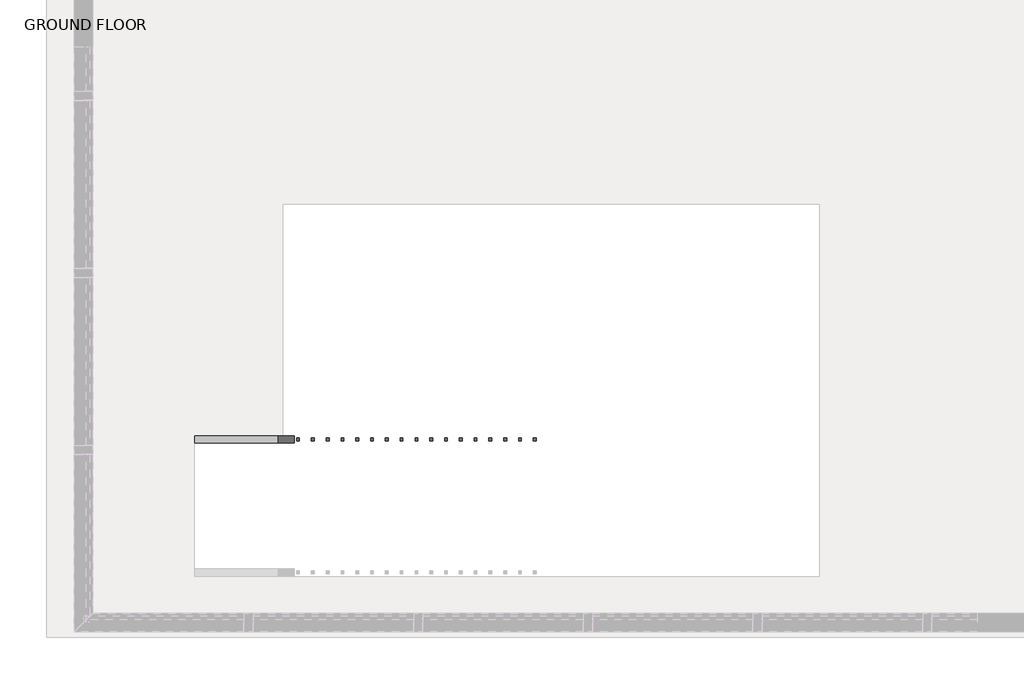
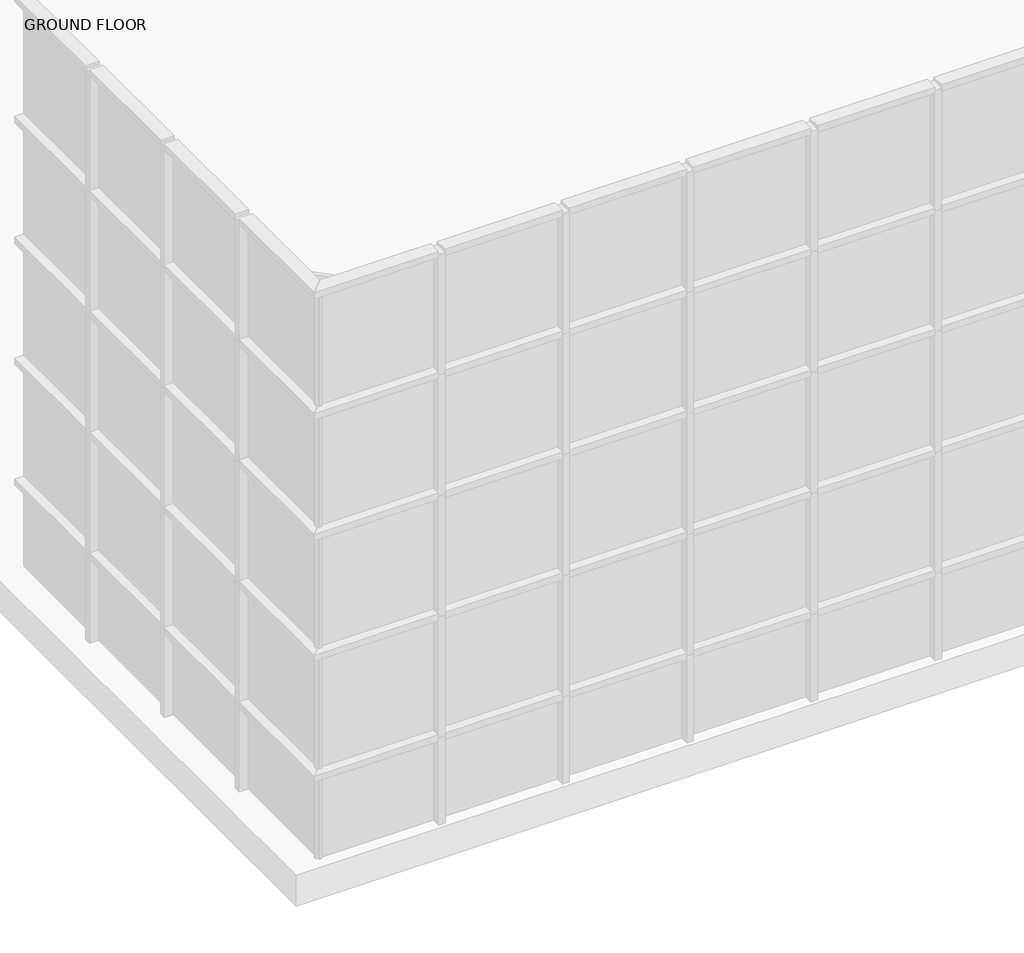
# One storey, part 16 of 16: 1 railing.
"""IFC4 building model written with IfcOpenShell, lengths in millimetres."""

from ifc_helpers import new_model, si_unit, frame, origin, place, context, project, spatial, polyline, outline, extrude, faceted_brep, element, save

model = new_model("IFC4")

# Units and contexts
model_context = context("Model", 3, world=origin())
ifc_project = project(units=[si_unit("LENGTHUNIT", "METRE", prefix="MILLI")], contexts=[model_context])

# Site, building, storey
site = spatial("IfcSite", under=ifc_project)
building = spatial("IfcBuilding", under=site)
storey = spatial("IfcBuildingStorey", under=building, Name="GROUND FLOOR", Elevation=0.0)

# Railing
placement = place(None, origin())
element("IfcRailing", 1, ObjectType="Handrail - Rectangular", at=placement, inside=storey, context=model_context, shape_type="SolidModel", body=[
    faceted_brep([(-8362.2800418, -4455.7090076, 914.4), (-8362.2800418, -4455.7090076, 857.6038734), (-8362.2800418, -4506.5090076, 857.6038734), (-8362.2800418, -4506.5090076, 914.4), (-5111.0800418, -4455.7090076, 2540.0), (-5060.2800418, -4455.7090076, 2508.6038734), (-5060.2800418, -4506.5090076, 2508.6038734), (-5111.0800418, -4506.5090076, 2540.0), (-5111.0800418, -4455.7090076, 2590.8), (-5060.2800418, -4455.7090076, 2540.0), (-5060.2800418, -4506.5090076, 2540.0), (-5111.0800418, -4506.5090076, 2590.8), (-5034.8800418, -4455.7090076, 2590.8), (-5034.8800418, -4455.7090076, 2540.0), (-4984.0800418, -4506.5090076, 2540.0), (-4984.0800418, -4506.5090076, 2590.8), (-5034.8800418, -4379.5090076, 2590.8), (-5034.8800418, -4379.5090076, 2540.0), (-4984.0800418, -4379.5090076, 2540.0), (-4984.0800418, -4379.5090076, 2590.8), (-5034.8800418, -3907.7346494, 2590.8), (-5034.8800418, -3856.9346494, 2540.0), (-4984.0800418, -3856.9346494, 2540.0), (-4984.0800418, -3907.7346494, 2590.8), (-5034.8800418, -3907.7346494, 2641.6), (-5034.8800418, -3856.9346494, 2590.8), (-4984.0800418, -3856.9346494, 2590.8), (-4984.0800418, -3907.7346494, 2641.6), (-5034.8800418, -3831.5346494, 2641.6), (-5034.8800418, -3831.5346494, 2590.8), (-4984.0800418, -3780.7346494, 2590.8), (-4984.0800418, -3780.7346494, 2641.6), (-5111.0800418, -3831.5346494, 2641.6), (-5123.072295, -3831.5346494, 2590.8), (-5123.072295, -3780.7346494, 2590.8), (-5111.0800418, -3780.7346494, 2641.6), (-7752.6800418, -3831.5346494, 3962.4), (-7752.6800418, -3780.7346494, 3962.4), (-7752.6800418, -3780.7346494, 3905.6038734), (-7752.6800418, -3831.5346494, 3905.6038734)], [[[0, 1, 2, 3]], [[1, 0, 4, 5]], [[2, 1, 5, 6]], [[3, 2, 6, 7]], [[0, 3, 7, 4]], [[5, 4, 8, 9]], [[6, 5, 9, 10]], [[7, 6, 10, 11]], [[4, 7, 11, 8]], [[9, 8, 12, 13]], [[10, 9, 13, 14]], [[11, 10, 14, 15]], [[8, 11, 15, 12]], [[13, 12, 16, 17]], [[14, 13, 17, 18]], [[15, 14, 18, 19]], [[12, 15, 19, 16]], [[17, 16, 20, 21]], [[18, 17, 21, 22]], [[19, 18, 22, 23]], [[16, 19, 23, 20]], [[21, 20, 24, 25]], [[22, 21, 25, 26]], [[23, 22, 26, 27]], [[20, 23, 27, 24]], [[25, 24, 28, 29]], [[26, 25, 29, 30]], [[27, 26, 30, 31]], [[24, 27, 31, 28]], [[29, 28, 32, 33]], [[30, 29, 33, 34]], [[31, 30, 34, 35]], [[28, 31, 35, 32]], [[36, 37, 38, 39]], [[33, 32, 36, 39]], [[34, 33, 39, 38]], [[35, 34, 38, 37]], [[32, 35, 37, 36]]]),
    extrude(outline(polyline([(3850.0413734, -7641.5550418), (3859.5663734, -7660.6050418), (3001.9625, -7660.6050418), (2992.4375, -7641.5550418), (3850.0413734, -7641.5550418)])), frame((0.0, -3815.6596494, 0.0), z_axis=(0.0, 1.0, 0.0), x_axis=(0.0, 0.0, 1.0)), (0.0, 0.0, 1.0), 19.05),
    extrude(outline(polyline([(3799.2413734, -7539.9550418), (3808.7663734, -7559.0050418), (2951.1625, -7559.0050418), (2941.6375, -7539.9550418), (3799.2413734, -7539.9550418)])), frame((0.0, -3815.6596494, 0.0), z_axis=(0.0, 1.0, 0.0), x_axis=(0.0, 0.0, 1.0)), (0.0, 0.0, 1.0), 19.05),
    extrude(outline(polyline([(3748.4413734, -7438.3550418), (3757.9663734, -7457.4050418), (2900.3625, -7457.4050418), (2890.8375, -7438.3550418), (3748.4413734, -7438.3550418)])), frame((0.0, -3815.6596494, 0.0), z_axis=(0.0, 1.0, 0.0), x_axis=(0.0, 0.0, 1.0)), (0.0, 0.0, 1.0), 19.05),
    extrude(outline(polyline([(3697.6413734, -7336.7550418), (3707.1663734, -7355.8050418), (2849.5625, -7355.8050418), (2840.0375, -7336.7550418), (3697.6413734, -7336.7550418)])), frame((0.0, -3815.6596494, 0.0), z_axis=(0.0, 1.0, 0.0), x_axis=(0.0, 0.0, 1.0)), (0.0, 0.0, 1.0), 19.05),
    extrude(outline(polyline([(3646.8413734, -7235.1550418), (3656.3663734, -7254.2050418), (2798.7625, -7254.2050418), (2789.2375, -7235.1550418), (3646.8413734, -7235.1550418)])), frame((0.0, -3815.6596494, 0.0), z_axis=(0.0, 1.0, 0.0), x_axis=(0.0, 0.0, 1.0)), (0.0, 0.0, 1.0), 19.05),
    extrude(outline(polyline([(3596.0413734, -7133.5550418), (3605.5663734, -7152.6050418), (2747.9625, -7152.6050418), (2738.4375, -7133.5550418), (3596.0413734, -7133.5550418)])), frame((0.0, -3815.6596494, 0.0), z_axis=(0.0, 1.0, 0.0), x_axis=(0.0, 0.0, 1.0)), (0.0, 0.0, 1.0), 19.05),
    extrude(outline(polyline([(3545.2413734, -7031.9550418), (3554.7663734, -7051.0050418), (2697.1625, -7051.0050418), (2687.6375, -7031.9550418), (3545.2413734, -7031.9550418)])), frame((0.0, -3815.6596494, 0.0), z_axis=(0.0, 1.0, 0.0), x_axis=(0.0, 0.0, 1.0)), (0.0, 0.0, 1.0), 19.05),
    extrude(outline(polyline([(3494.4413734, -6930.3550418), (3503.9663734, -6949.4050418), (2646.3625, -6949.4050418), (2636.8375, -6930.3550418), (3494.4413734, -6930.3550418)])), frame((0.0, -3815.6596494, 0.0), z_axis=(0.0, 1.0, 0.0), x_axis=(0.0, 0.0, 1.0)), (0.0, 0.0, 1.0), 19.05),
    extrude(outline(polyline([(3443.6413734, -6828.7550418), (3453.1663734, -6847.8050418), (2595.5625, -6847.8050418), (2586.0375, -6828.7550418), (3443.6413734, -6828.7550418)])), frame((0.0, -3815.6596494, 0.0), z_axis=(0.0, 1.0, 0.0), x_axis=(0.0, 0.0, 1.0)), (0.0, 0.0, 1.0), 19.05),
    extrude(outline(polyline([(3392.8413734, -6727.1550418), (3402.3663734, -6746.2050418), (2544.7625, -6746.2050418), (2535.2375, -6727.1550418), (3392.8413734, -6727.1550418)])), frame((0.0, -3815.6596494, 0.0), z_axis=(0.0, 1.0, 0.0), x_axis=(0.0, 0.0, 1.0)), (0.0, 0.0, 1.0), 19.05),
    extrude(outline(polyline([(3342.0413734, -6625.5550418), (3351.5663734, -6644.6050418), (2493.9625, -6644.6050418), (2484.4375, -6625.5550418), (3342.0413734, -6625.5550418)])), frame((0.0, -3815.6596494, 0.0), z_axis=(0.0, 1.0, 0.0), x_axis=(0.0, 0.0, 1.0)), (0.0, 0.0, 1.0), 19.05),
    extrude(outline(polyline([(3291.2413734, -6523.9550418), (3300.7663734, -6543.0050418), (2443.1625, -6543.0050418), (2433.6375, -6523.9550418), (3291.2413734, -6523.9550418)])), frame((0.0, -3815.6596494, 0.0), z_axis=(0.0, 1.0, 0.0), x_axis=(0.0, 0.0, 1.0)), (0.0, 0.0, 1.0), 19.05),
    extrude(outline(polyline([(3240.4413734, -6422.3550418), (3249.9663734, -6441.4050418), (2392.3625, -6441.4050418), (2382.8375, -6422.3550418), (3240.4413734, -6422.3550418)])), frame((0.0, -3815.6596494, 0.0), z_axis=(0.0, 1.0, 0.0), x_axis=(0.0, 0.0, 1.0)), (0.0, 0.0, 1.0), 19.05),
    extrude(outline(polyline([(3189.6413734, -6320.7550418), (3199.1663734, -6339.8050418), (2341.5625, -6339.8050418), (2332.0375, -6320.7550418), (3189.6413734, -6320.7550418)])), frame((0.0, -3815.6596494, 0.0), z_axis=(0.0, 1.0, 0.0), x_axis=(0.0, 0.0, 1.0)), (0.0, 0.0, 1.0), 19.05),
    extrude(outline(polyline([(3138.8413734, -6219.1550418), (3148.3663734, -6238.2050418), (2290.7625, -6238.2050418), (2281.2375, -6219.1550418), (3138.8413734, -6219.1550418)])), frame((0.0, -3815.6596494, 0.0), z_axis=(0.0, 1.0, 0.0), x_axis=(0.0, 0.0, 1.0)), (0.0, 0.0, 1.0), 19.05),
    extrude(outline(polyline([(3088.0413734, -6117.5550418), (3097.5663734, -6136.6050418), (2239.9625, -6136.6050418), (2230.4375, -6117.5550418), (3088.0413734, -6117.5550418)])), frame((0.0, -3815.6596494, 0.0), z_axis=(0.0, 1.0, 0.0), x_axis=(0.0, 0.0, 1.0)), (0.0, 0.0, 1.0), 19.05),
    extrude(outline(polyline([(3037.2413734, -6015.9550418), (3046.7663734, -6035.0050418), (2189.1625, -6035.0050418), (2179.6375, -6015.9550418), (3037.2413734, -6015.9550418)])), frame((0.0, -3815.6596494, 0.0), z_axis=(0.0, 1.0, 0.0), x_axis=(0.0, 0.0, 1.0)), (0.0, 0.0, 1.0), 19.05),
    extrude(outline(polyline([(2986.4413734, -5914.3550418), (2995.9663734, -5933.4050418), (2138.3625, -5933.4050418), (2128.8375, -5914.3550418), (2986.4413734, -5914.3550418)])), frame((0.0, -3815.6596494, 0.0), z_axis=(0.0, 1.0, 0.0), x_axis=(0.0, 0.0, 1.0)), (0.0, 0.0, 1.0), 19.05),
    extrude(outline(polyline([(2935.6413734, -5812.7550418), (2945.1663734, -5831.8050418), (2087.5625, -5831.8050418), (2078.0375, -5812.7550418), (2935.6413734, -5812.7550418)])), frame((0.0, -3815.6596494, 0.0), z_axis=(0.0, 1.0, 0.0), x_axis=(0.0, 0.0, 1.0)), (0.0, 0.0, 1.0), 19.05),
    extrude(outline(polyline([(2884.8413734, -5711.1550418), (2894.3663734, -5730.2050418), (2036.7625, -5730.2050418), (2027.2375, -5711.1550418), (2884.8413734, -5711.1550418)])), frame((0.0, -3815.6596494, 0.0), z_axis=(0.0, 1.0, 0.0), x_axis=(0.0, 0.0, 1.0)), (0.0, 0.0, 1.0), 19.05),
    extrude(outline(polyline([(2834.0413734, -5609.5550418), (2843.5663734, -5628.6050418), (1985.9625, -5628.6050418), (1976.4375, -5609.5550418), (2834.0413734, -5609.5550418)])), frame((0.0, -3815.6596494, 0.0), z_axis=(0.0, 1.0, 0.0), x_axis=(0.0, 0.0, 1.0)), (0.0, 0.0, 1.0), 19.05),
    extrude(outline(polyline([(2783.2413734, -5507.9550418), (2792.7663734, -5527.0050418), (1935.1625, -5527.0050418), (1925.6375, -5507.9550418), (2783.2413734, -5507.9550418)])), frame((0.0, -3815.6596494, 0.0), z_axis=(0.0, 1.0, 0.0), x_axis=(0.0, 0.0, 1.0)), (0.0, 0.0, 1.0), 19.05),
    extrude(outline(polyline([(2732.4413734, -5406.3550418), (2741.9663734, -5425.4050418), (1884.3625, -5425.4050418), (1874.8375, -5406.3550418), (2732.4413734, -5406.3550418)])), frame((0.0, -3815.6596494, 0.0), z_axis=(0.0, 1.0, 0.0), x_axis=(0.0, 0.0, 1.0)), (0.0, 0.0, 1.0), 19.05),
    extrude(outline(polyline([(2681.6413734, -5304.7550418), (2691.1663734, -5323.8050418), (1833.5625, -5323.8050418), (1824.0375, -5304.7550418), (2681.6413734, -5304.7550418)])), frame((0.0, -3815.6596494, 0.0), z_axis=(0.0, 1.0, 0.0), x_axis=(0.0, 0.0, 1.0)), (0.0, 0.0, 1.0), 19.05),
    extrude(outline(polyline([(2630.8413734, -5203.1550418), (2640.3663734, -5222.2050418), (1782.7625, -5222.2050418), (1773.2375, -5203.1550418), (2630.8413734, -5203.1550418)])), frame((0.0, -3815.6596494, 0.0), z_axis=(0.0, 1.0, 0.0), x_axis=(0.0, 0.0, 1.0)), (0.0, 0.0, 1.0), 19.05),
    extrude(outline(polyline([(2590.8, -5101.5550418), (2590.8, -5120.6050418), (1731.9625, -5120.6050418), (1722.4375, -5101.5550418), (2590.8, -5101.5550418)])), frame((0.0, -3815.6596494, 0.0), z_axis=(0.0, 1.0, 0.0), x_axis=(0.0, 0.0, 1.0)), (0.0, 0.0, 1.0), 19.05),
    extrude(outline(polyline([(-4999.9550418, -3881.0340076), (-5019.0050418, -3881.0340076), (-5019.0050418, -3861.9840076), (-4999.9550418, -3861.9840076), (-4999.9550418, -3881.0340076)])), frame((0.0, 0.0, 1676.4), z_axis=(0.0, 0.0, 1.0), x_axis=(1.0, 0.0, 0.0)), (0.0, 0.0, 1.0), 863.6),
    extrude(outline(polyline([(-4999.9550418, -3982.6340076), (-5019.0050418, -3982.6340076), (-5019.0050418, -3963.5840076), (-4999.9550418, -3963.5840076), (-4999.9550418, -3982.6340076)])), frame((0.0, 0.0, 1676.4), z_axis=(0.0, 0.0, 1.0), x_axis=(1.0, 0.0, 0.0)), (0.0, 0.0, 1.0), 863.6),
    extrude(outline(polyline([(-4999.9550418, -4084.2340076), (-5019.0050418, -4084.2340076), (-5019.0050418, -4065.1840076), (-4999.9550418, -4065.1840076), (-4999.9550418, -4084.2340076)])), frame((0.0, 0.0, 1676.4), z_axis=(0.0, 0.0, 1.0), x_axis=(1.0, 0.0, 0.0)), (0.0, 0.0, 1.0), 863.6),
    extrude(outline(polyline([(-4999.9550418, -4185.8340076), (-5019.0050418, -4185.8340076), (-5019.0050418, -4166.7840076), (-4999.9550418, -4166.7840076), (-4999.9550418, -4185.8340076)])), frame((0.0, 0.0, 1676.4), z_axis=(0.0, 0.0, 1.0), x_axis=(1.0, 0.0, 0.0)), (0.0, 0.0, 1.0), 863.6),
    extrude(outline(polyline([(-4999.9550418, -4287.4340076), (-5019.0050418, -4287.4340076), (-5019.0050418, -4268.3840076), (-4999.9550418, -4268.3840076), (-4999.9550418, -4287.4340076)])), frame((0.0, 0.0, 1676.4), z_axis=(0.0, 0.0, 1.0), x_axis=(1.0, 0.0, 0.0)), (0.0, 0.0, 1.0), 863.6),
    extrude(outline(polyline([(-4999.9550418, -4389.0340076), (-5019.0050418, -4389.0340076), (-5019.0050418, -4369.9840076), (-4999.9550418, -4369.9840076), (-4999.9550418, -4389.0340076)])), frame((0.0, 0.0, 1676.4), z_axis=(0.0, 0.0, 1.0), x_axis=(1.0, 0.0, 0.0)), (0.0, 0.0, 1.0), 863.6),
    extrude(outline(polyline([(2487.9663734, -5101.5550418), (2478.4413734, -5120.6050418), (1620.8375, -5120.6050418), (1630.3625, -5101.5550418), (2487.9663734, -5101.5550418)])), frame((0.0, -4490.6340076, 0.0), z_axis=(0.0, 1.0, 0.0), x_axis=(0.0, 0.0, 1.0)), (0.0, 0.0, 1.0), 19.05),
    extrude(outline(polyline([(2437.1663734, -5203.1550418), (2427.6413734, -5222.2050418), (1570.0375, -5222.2050418), (1579.5625, -5203.1550418), (2437.1663734, -5203.1550418)])), frame((0.0, -4490.6340076, 0.0), z_axis=(0.0, 1.0, 0.0), x_axis=(0.0, 0.0, 1.0)), (0.0, 0.0, 1.0), 19.05),
    extrude(outline(polyline([(2386.3663734, -5304.7550418), (2376.8413734, -5323.8050418), (1519.2375, -5323.8050418), (1528.7625, -5304.7550418), (2386.3663734, -5304.7550418)])), frame((0.0, -4490.6340076, 0.0), z_axis=(0.0, 1.0, 0.0), x_axis=(0.0, 0.0, 1.0)), (0.0, 0.0, 1.0), 19.05),
    extrude(outline(polyline([(2335.5663734, -5406.3550418), (2326.0413734, -5425.4050418), (1468.4375, -5425.4050418), (1477.9625, -5406.3550418), (2335.5663734, -5406.3550418)])), frame((0.0, -4490.6340076, 0.0), z_axis=(0.0, 1.0, 0.0), x_axis=(0.0, 0.0, 1.0)), (0.0, 0.0, 1.0), 19.05),
    extrude(outline(polyline([(2284.7663734, -5507.9550418), (2275.2413734, -5527.0050418), (1417.6375, -5527.0050418), (1427.1625, -5507.9550418), (2284.7663734, -5507.9550418)])), frame((0.0, -4490.6340076, 0.0), z_axis=(0.0, 1.0, 0.0), x_axis=(0.0, 0.0, 1.0)), (0.0, 0.0, 1.0), 19.05),
    extrude(outline(polyline([(2233.9663734, -5609.5550418), (2224.4413734, -5628.6050418), (1366.8375, -5628.6050418), (1376.3625, -5609.5550418), (2233.9663734, -5609.5550418)])), frame((0.0, -4490.6340076, 0.0), z_axis=(0.0, 1.0, 0.0), x_axis=(0.0, 0.0, 1.0)), (0.0, 0.0, 1.0), 19.05),
    extrude(outline(polyline([(2183.1663734, -5711.1550418), (2173.6413734, -5730.2050418), (1316.0375, -5730.2050418), (1325.5625, -5711.1550418), (2183.1663734, -5711.1550418)])), frame((0.0, -4490.6340076, 0.0), z_axis=(0.0, 1.0, 0.0), x_axis=(0.0, 0.0, 1.0)), (0.0, 0.0, 1.0), 19.05),
    extrude(outline(polyline([(2132.3663734, -5812.7550418), (2122.8413734, -5831.8050418), (1265.2375, -5831.8050418), (1274.7625, -5812.7550418), (2132.3663734, -5812.7550418)])), frame((0.0, -4490.6340076, 0.0), z_axis=(0.0, 1.0, 0.0), x_axis=(0.0, 0.0, 1.0)), (0.0, 0.0, 1.0), 19.05),
    extrude(outline(polyline([(2081.5663734, -5914.3550418), (2072.0413734, -5933.4050418), (1214.4375, -5933.4050418), (1223.9625, -5914.3550418), (2081.5663734, -5914.3550418)])), frame((0.0, -4490.6340076, 0.0), z_axis=(0.0, 1.0, 0.0), x_axis=(0.0, 0.0, 1.0)), (0.0, 0.0, 1.0), 19.05),
    extrude(outline(polyline([(2030.7663734, -6015.9550418), (2021.2413734, -6035.0050418), (1163.6375, -6035.0050418), (1173.1625, -6015.9550418), (2030.7663734, -6015.9550418)])), frame((0.0, -4490.6340076, 0.0), z_axis=(0.0, 1.0, 0.0), x_axis=(0.0, 0.0, 1.0)), (0.0, 0.0, 1.0), 19.05),
    extrude(outline(polyline([(1979.9663734, -6117.5550418), (1970.4413734, -6136.6050418), (1112.8375, -6136.6050418), (1122.3625, -6117.5550418), (1979.9663734, -6117.5550418)])), frame((0.0, -4490.6340076, 0.0), z_axis=(0.0, 1.0, 0.0), x_axis=(0.0, 0.0, 1.0)), (0.0, 0.0, 1.0), 19.05),
    extrude(outline(polyline([(1929.1663734, -6219.1550418), (1919.6413734, -6238.2050418), (1062.0375, -6238.2050418), (1071.5625, -6219.1550418), (1929.1663734, -6219.1550418)])), frame((0.0, -4490.6340076, 0.0), z_axis=(0.0, 1.0, 0.0), x_axis=(0.0, 0.0, 1.0)), (0.0, 0.0, 1.0), 19.05),
    extrude(outline(polyline([(1878.3663734, -6320.7550418), (1868.8413734, -6339.8050418), (1011.2375, -6339.8050418), (1020.7625, -6320.7550418), (1878.3663734, -6320.7550418)])), frame((0.0, -4490.6340076, 0.0), z_axis=(0.0, 1.0, 0.0), x_axis=(0.0, 0.0, 1.0)), (0.0, 0.0, 1.0), 19.05),
    extrude(outline(polyline([(1827.5663734, -6422.3550418), (1818.0413734, -6441.4050418), (960.4375, -6441.4050418), (969.9625, -6422.3550418), (1827.5663734, -6422.3550418)])), frame((0.0, -4490.6340076, 0.0), z_axis=(0.0, 1.0, 0.0), x_axis=(0.0, 0.0, 1.0)), (0.0, 0.0, 1.0), 19.05),
    extrude(outline(polyline([(1776.7663734, -6523.9550418), (1767.2413734, -6543.0050418), (909.6375, -6543.0050418), (919.1625, -6523.9550418), (1776.7663734, -6523.9550418)])), frame((0.0, -4490.6340076, 0.0), z_axis=(0.0, 1.0, 0.0), x_axis=(0.0, 0.0, 1.0)), (0.0, 0.0, 1.0), 19.05),
    extrude(outline(polyline([(1725.9663734, -6625.5550418), (1716.4413734, -6644.6050418), (858.8375, -6644.6050418), (868.3625, -6625.5550418), (1725.9663734, -6625.5550418)])), frame((0.0, -4490.6340076, 0.0), z_axis=(0.0, 1.0, 0.0), x_axis=(0.0, 0.0, 1.0)), (0.0, 0.0, 1.0), 19.05),
    extrude(outline(polyline([(1675.1663734, -6727.1550418), (1665.6413734, -6746.2050418), (808.0375, -6746.2050418), (817.5625, -6727.1550418), (1675.1663734, -6727.1550418)])), frame((0.0, -4490.6340076, 0.0), z_axis=(0.0, 1.0, 0.0), x_axis=(0.0, 0.0, 1.0)), (0.0, 0.0, 1.0), 19.05),
    extrude(outline(polyline([(1624.3663734, -6828.7550418), (1614.8413734, -6847.8050418), (757.2375, -6847.8050418), (766.7625, -6828.7550418), (1624.3663734, -6828.7550418)])), frame((0.0, -4490.6340076, 0.0), z_axis=(0.0, 1.0, 0.0), x_axis=(0.0, 0.0, 1.0)), (0.0, 0.0, 1.0), 19.05),
    extrude(outline(polyline([(1573.5663734, -6930.3550418), (1564.0413734, -6949.4050418), (706.4375, -6949.4050418), (715.9625, -6930.3550418), (1573.5663734, -6930.3550418)])), frame((0.0, -4490.6340076, 0.0), z_axis=(0.0, 1.0, 0.0), x_axis=(0.0, 0.0, 1.0)), (0.0, 0.0, 1.0), 19.05),
    extrude(outline(polyline([(1522.7663734, -7031.9550418), (1513.2413734, -7051.0050418), (655.6375, -7051.0050418), (665.1625, -7031.9550418), (1522.7663734, -7031.9550418)])), frame((0.0, -4490.6340076, 0.0), z_axis=(0.0, 1.0, 0.0), x_axis=(0.0, 0.0, 1.0)), (0.0, 0.0, 1.0), 19.05),
    extrude(outline(polyline([(1471.9663734, -7133.5550418), (1462.4413734, -7152.6050418), (604.8375, -7152.6050418), (614.3625, -7133.5550418), (1471.9663734, -7133.5550418)])), frame((0.0, -4490.6340076, 0.0), z_axis=(0.0, 1.0, 0.0), x_axis=(0.0, 0.0, 1.0)), (0.0, 0.0, 1.0), 19.05),
    extrude(outline(polyline([(1421.1663734, -7235.1550418), (1411.6413734, -7254.2050418), (554.0375, -7254.2050418), (563.5625, -7235.1550418), (1421.1663734, -7235.1550418)])), frame((0.0, -4490.6340076, 0.0), z_axis=(0.0, 1.0, 0.0), x_axis=(0.0, 0.0, 1.0)), (0.0, 0.0, 1.0), 19.05),
    extrude(outline(polyline([(1370.3663734, -7336.7550418), (1360.8413734, -7355.8050418), (503.2375, -7355.8050418), (512.7625, -7336.7550418), (1370.3663734, -7336.7550418)])), frame((0.0, -4490.6340076, 0.0), z_axis=(0.0, 1.0, 0.0), x_axis=(0.0, 0.0, 1.0)), (0.0, 0.0, 1.0), 19.05),
    extrude(outline(polyline([(1319.5663734, -7438.3550418), (1310.0413734, -7457.4050418), (452.4375, -7457.4050418), (461.9625, -7438.3550418), (1319.5663734, -7438.3550418)])), frame((0.0, -4490.6340076, 0.0), z_axis=(0.0, 1.0, 0.0), x_axis=(0.0, 0.0, 1.0)), (0.0, 0.0, 1.0), 19.05),
    extrude(outline(polyline([(1268.7663734, -7539.9550418), (1259.2413734, -7559.0050418), (401.6375, -7559.0050418), (411.1625, -7539.9550418), (1268.7663734, -7539.9550418)])), frame((0.0, -4490.6340076, 0.0), z_axis=(0.0, 1.0, 0.0), x_axis=(0.0, 0.0, 1.0)), (0.0, 0.0, 1.0), 19.05),
    extrude(outline(polyline([(1217.9663734, -7641.5550418), (1208.4413734, -7660.6050418), (350.8375, -7660.6050418), (360.3625, -7641.5550418), (1217.9663734, -7641.5550418)])), frame((0.0, -4490.6340076, 0.0), z_axis=(0.0, 1.0, 0.0), x_axis=(0.0, 0.0, 1.0)), (0.0, 0.0, 1.0), 19.05),
    extrude(outline(polyline([(1167.1663734, -7743.1550418), (1157.6413734, -7762.2050418), (300.0375, -7762.2050418), (309.5625, -7743.1550418), (1167.1663734, -7743.1550418)])), frame((0.0, -4490.6340076, 0.0), z_axis=(0.0, 1.0, 0.0), x_axis=(0.0, 0.0, 1.0)), (0.0, 0.0, 1.0), 19.05),
    extrude(outline(polyline([(1116.3663734, -7844.7550418), (1106.8413734, -7863.8050418), (249.2375, -7863.8050418), (258.7625, -7844.7550418), (1116.3663734, -7844.7550418)])), frame((0.0, -4490.6340076, 0.0), z_axis=(0.0, 1.0, 0.0), x_axis=(0.0, 0.0, 1.0)), (0.0, 0.0, 1.0), 19.05),
    extrude(outline(polyline([(1065.5663734, -7946.3550418), (1056.0413734, -7965.4050418), (198.4375, -7965.4050418), (207.9625, -7946.3550418), (1065.5663734, -7946.3550418)])), frame((0.0, -4490.6340076, 0.0), z_axis=(0.0, 1.0, 0.0), x_axis=(0.0, 0.0, 1.0)), (0.0, 0.0, 1.0), 19.05),
    extrude(outline(polyline([(1014.7663734, -8047.9550418), (1005.2413734, -8067.0050418), (147.6375, -8067.0050418), (157.1625, -8047.9550418), (1014.7663734, -8047.9550418)])), frame((0.0, -4490.6340076, 0.0), z_axis=(0.0, 1.0, 0.0), x_axis=(0.0, 0.0, 1.0)), (0.0, 0.0, 1.0), 19.05),
    extrude(outline(polyline([(963.9663734, -8149.5550418), (954.4413734, -8168.6050418), (96.8375, -8168.6050418), (106.3625, -8149.5550418), (963.9663734, -8149.5550418)])), frame((0.0, -4490.6340076, 0.0), z_axis=(0.0, 1.0, 0.0), x_axis=(0.0, 0.0, 1.0)), (0.0, 0.0, 1.0), 19.05),
    extrude(outline(polyline([(913.1663734, -8251.1550418), (903.6413734, -8270.2050418), (46.0375, -8270.2050418), (55.5625, -8251.1550418), (913.1663734, -8251.1550418)])), frame((0.0, -4490.6340076, 0.0), z_axis=(0.0, 1.0, 0.0), x_axis=(0.0, 0.0, 1.0)), (0.0, 0.0, 1.0), 19.05),
    extrude(outline(polyline([(-4999.9550418, -3815.6596494), (-5019.0050418, -3815.6596494), (-5019.0050418, -3796.6096494), (-4999.9550418, -3796.6096494), (-4999.9550418, -3815.6596494)])), frame((0.0, 0.0, 1676.4), z_axis=(0.0, 0.0, 1.0), x_axis=(1.0, 0.0, 0.0)), (0.0, 0.0, 1.0), 914.4),
    extrude(outline(polyline([(2540.0, -4999.9550418), (2540.0, -5019.0050418), (1671.6375, -5019.0050418), (1681.1625, -4999.9550418), (2540.0, -4999.9550418)])), frame((0.0, -4490.6340076, 0.0), z_axis=(0.0, 1.0, 0.0), x_axis=(0.0, 0.0, 1.0)), (0.0, 0.0, 1.0), 19.05),
    extrude(outline(polyline([(3896.0788734, -7733.6300418), (3905.6038734, -7752.6800418), (3048.0, -7752.6800418), (3038.475, -7733.6300418), (3896.0788734, -7733.6300418)])), frame((0.0, -3815.6596494, 0.0), z_axis=(0.0, 1.0, 0.0), x_axis=(0.0, 0.0, 1.0)), (0.0, 0.0, 1.0), 19.05),
    extrude(outline(polyline([(867.1288734, -8343.2300418), (857.6038734, -8362.2800418), (0.0, -8362.2800418), (9.525, -8343.2300418), (867.1288734, -8343.2300418)])), frame((0.0, -4490.6340076, 0.0), z_axis=(0.0, 1.0, 0.0), x_axis=(0.0, 0.0, 1.0)), (0.0, 0.0, 1.0), 19.05),
])

save(model, "model.ifc")

# Revit data of these elements
# Type "Handrail - Rectangular"
#   Assembly Code = "C2010400"
#   built-in parameter 1008612 = 0.0416667 (stored number, unit not read)
#   built-in parameter 1008611 = 0.0416667 (stored number, unit not read)
#   built-in parameter 1008609 = 0.333333 (stored number, unit not read)
#   built-in parameter 1008604 = 0.166667 (stored number, unit not read)
#   built-in parameter 1008603 = 0.166667 (stored number, unit not read)
#   Railing Height = 3' - 0"
#   built-in parameter 1008630 = 2
#   built-in parameter 1008610 = 2
#   built-in parameter 1008618 = Baluster - Square : 3/4"
# Element 1 (IfcRailing, "Handrail - Rectangular")
#   Phase Created = New Construction
